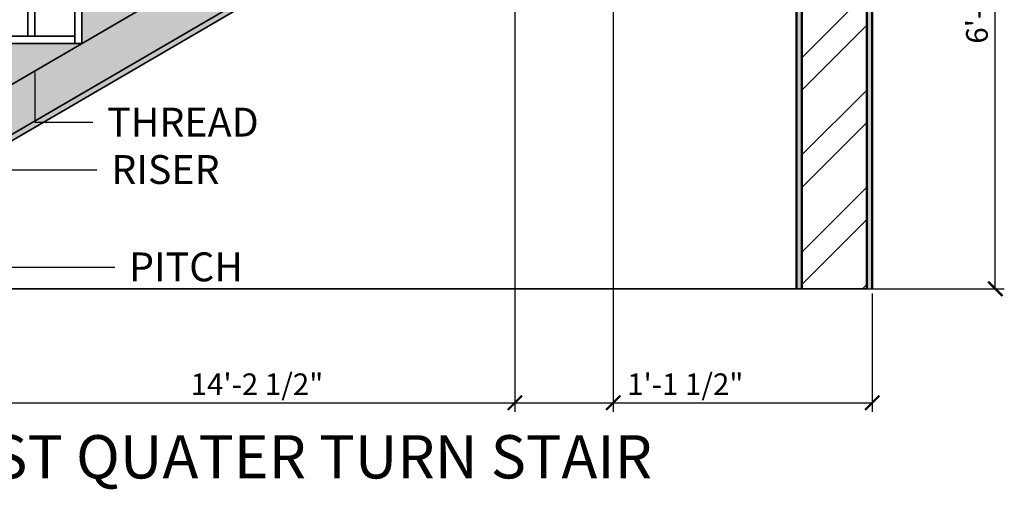
# Model space of a CAD drawing. Units: inches. Extents: x 2205 to 2524, y 4609 to 4803.
# Tile 2 of 5: x 2311 to 2447, y 4609 to 4674. Entities that reach past the tile are written whole.
import ezdxf
from ezdxf import colors
from ezdxf.entities.mleader import LeaderData, LeaderLine
from ezdxf.math import Vec2, Vec3

# ---------------------------------------------------------------- set-up
doc = ezdxf.new("R2010")
doc.units = ezdxf.units.IN
for name, color, linetype, lineweight in [('A-ANNO-DIMS', 2, 'Continuous', 18), ('A-ANNO-SYMB', 3, 'Continuous', 18), ('A-ANNO-TEXT', 7, 'Continuous', 18), ('A-FLOR-STRS', 7, 'Continuous', 35), ('A-SECT', 7, 'Continuous', 25), ('A-SECT-PATT', 252, 'Continuous', 13), ('A-WALL', 1, 'Continuous', 50), ('A-WALL-PATT', 8, 'Continuous', 13)]:
    doc.layers.add(name, color=color, linetype=linetype, lineweight=lineweight)
doc.styles.get("Standard").update_dxf_attribs({"font": 'arial.ttf'})
doc.dimstyles.new('ISO-25', dxfattribs={"dimtxt": 3, "dimasz": 2, "dimexe": 1.25, "dimexo": 0.625, "dimtad": 1, "dimdec": 1, "dimlunit": 3, "dimtxsty": 'Standard', "dimblk": 'ARCHTICK', "dimcen": 2.5, "dimclrd": 5, "dimclre": 2, "dimclrt": 6, "dimadec": 0, "dimazin": 0, "dimtfac": 1, "dimtdec": 1, "dimtmove": 0, "dimatfit": 3, "dimfxl": 1, "dimarcsym": 0})

# ---------------------------------------------------------------- blocks, each defined once
blk = doc.blocks.new('STAIR-STEP')
for p, q in [((2282.7, 4650.98), (2270.7, 4650.98)), ((2283.7, 4649.98), (2270.7, 4649.98)), ((2270.7, 4649.98), (2270.7, 4642.98)), ((2271.7, 4649.98), (2271.7, 4642.98))]:
    blk.add_line(p, q)
blk.add_arc((2270.7, 4650.48), 0.5, 90, 270)
blk = doc.blocks.new('BALUSTER')
for p, q in [((2276.2, 4684.66), (2276.2, 4650.98)), ((2277.2, 4685.25), (2277.2, 4650.98))]:
    blk.add_line(p, q)
blk = doc.blocks.new('_ArchTick')
at = {"color": 0, "linetype": 'ByBlock', "const_width": 0.15}
blk.add_lwpolyline([(-0.5, -0.5), (0.5, 0.5)], dxfattribs=at)
blk = doc.blocks.new('*D15')
at = {"layer": 'A-ANNO-DIMS', "color": 2, "lineweight": -2, "transparency": 16777216}
for p, q in [((2258.7, 4636.35), (2258.7, 4619.93)), ((2429.2, 4636.35), (2429.2, 4619.93))]:
    blk.add_line(p, q, dxfattribs=at)
at = {"layer": 'A-ANNO-DIMS', "color": 5, "lineweight": -2, "transparency": 16777216}
blk.add_line((2258.7, 4621.18), (2429.2, 4621.18), dxfattribs=at)
at = {"layer": 'DEFPOINTS', "color": 0, "transparency": 16777216}
for p in [(2258.7, 4636.98), (2429.2, 4636.98), (2429.2, 4621.18)]:
    blk.add_point(p, dxfattribs=at)
at = {"layer": 'A-ANNO-DIMS', "color": 5, "lineweight": -2, "transparency": 16777216, "xscale": 2, "yscale": 2, "zscale": 2, "rotation": 180}
blk.add_blockref('_ArchTick', (2258.7, 4621.18), dxfattribs=at)
at = {"layer": 'A-ANNO-DIMS', "color": 5, "lineweight": -2, "transparency": 16777216, "xscale": 2, "yscale": 2, "zscale": 2}
blk.add_blockref('_ArchTick', (2429.2, 4621.18), dxfattribs=at)
at = {"layer": 'A-ANNO-DIMS', "color": 6, "transparency": 16777216, "insert": (2343.95, 4623.36), "char_height": 3, "attachment_point": 5}
blk.add_mtext('14\'-2 1/2"', dxfattribs=at)
blk = doc.blocks.new('*D16')
at = {"layer": 'A-ANNO-DIMS', "color": 2, "lineweight": -2, "transparency": 16777216}
for p, q in [((2428.57, 4771.26), (2222.09, 4771.26)), ((2428.57, 4636.98), (2222.09, 4636.98))]:
    blk.add_line(p, q, dxfattribs=at)
at = {"layer": 'A-ANNO-DIMS', "color": 5, "lineweight": -2, "transparency": 16777216}
blk.add_line((2223.34, 4636.98), (2223.34, 4771.26), dxfattribs=at)
at = {"layer": 'DEFPOINTS', "color": 0, "transparency": 16777216}
for p in [(2223.34, 4771.26), (2429.2, 4771.26), (2429.2, 4636.98)]:
    blk.add_point(p, dxfattribs=at)
at = {"layer": 'A-ANNO-DIMS', "color": 5, "lineweight": -2, "transparency": 16777216, "xscale": 2, "yscale": 2, "zscale": 2}
for p, rotation in [((2223.34, 4771.26), 90), ((2223.34, 4636.98), 270)]:
    blk.add_blockref('_ArchTick', p, dxfattribs=dict(at, rotation=rotation))
at = {"layer": 'A-ANNO-DIMS', "color": 6, "transparency": 16777216, "insert": (2221.17, 4704.12), "char_height": 3, "attachment_point": 5, "rotation": 90}
blk.add_mtext('11\'-2 1/2"', dxfattribs=at)
blk = doc.blocks.new('*D17')
at = {"layer": 'A-ANNO-DIMS', "color": 2, "lineweight": -2, "transparency": 16777216}
for p, q in [((2420.07, 4713.98), (2447.5, 4713.98)), ((2420.07, 4636.98), (2447.5, 4636.98))]:
    blk.add_line(p, q, dxfattribs=at)
at = {"layer": 'A-ANNO-DIMS', "color": 5, "lineweight": -2, "transparency": 16777216}
blk.add_line((2446.25, 4636.98), (2446.25, 4713.98), dxfattribs=at)
at = {"layer": 'DEFPOINTS', "color": 0, "transparency": 16777216}
for p in [(2419.45, 4713.98), (2446.25, 4713.98), (2419.45, 4636.98)]:
    blk.add_point(p, dxfattribs=at)
at = {"layer": 'A-ANNO-DIMS', "color": 5, "lineweight": -2, "transparency": 16777216, "xscale": 2, "yscale": 2, "zscale": 2}
for p, rotation in [((2446.25, 4713.98), 90), ((2446.25, 4636.98), 270)]:
    blk.add_blockref('_ArchTick', p, dxfattribs=dict(at, rotation=rotation))
at = {"layer": 'A-ANNO-DIMS', "color": 6, "transparency": 16777216, "insert": (2444.09, 4675.48), "char_height": 3, "attachment_point": 5, "rotation": 90}
blk.add_mtext('6\'-5"', dxfattribs=at)
blk = doc.blocks.new('*D21')
at = {"layer": 'A-ANNO-DIMS', "color": 2, "lineweight": -2, "transparency": 16777216}
for p, q in [((2379.7, 4705.35), (2379.7, 4619.93)), ((2393.32, 4706.35), (2393.32, 4619.93))]:
    blk.add_line(p, q, dxfattribs=at)
at = {"layer": 'A-ANNO-DIMS', "color": 5, "lineweight": -2, "transparency": 16777216}
for p, q in [((2379.7, 4621.18), (2393.32, 4621.18)), ((2393.32, 4621.18), (2411.25, 4621.18))]:
    blk.add_line(p, q, dxfattribs=at)
at = {"layer": 'DEFPOINTS', "color": 0, "transparency": 16777216}
for p in [(2393.32, 4706.98), (2379.7, 4705.98), (2393.32, 4621.18)]:
    blk.add_point(p, dxfattribs=at)
at = {"layer": 'A-ANNO-DIMS', "color": 5, "lineweight": -2, "transparency": 16777216, "xscale": 2, "yscale": 2, "zscale": 2, "rotation": 180}
blk.add_blockref('_ArchTick', (2379.7, 4621.18), dxfattribs=at)
at = {"layer": 'A-ANNO-DIMS', "color": 5, "lineweight": -2, "transparency": 16777216, "xscale": 2, "yscale": 2, "zscale": 2}
blk.add_blockref('_ArchTick', (2393.32, 4621.18), dxfattribs=at)
at = {"layer": 'A-ANNO-DIMS', "color": 6, "transparency": 16777216, "insert": (2403.29, 4623.36), "char_height": 3, "attachment_point": 5}
blk.add_mtext('1\'-1 1/2"', dxfattribs=at)

msp = doc.modelspace()

# ---------------------------------------------------------------- hatches: boundary and pattern name
at = {"layer": 'A-SECT-PATT'}
h = msp.add_hatch(dxfattribs=at)
h.set_pattern_fill('AR-CONC', color=256, scale=0.04)
h.paths.add_polyline_path([(2393.32, 4706.98), (2419.45, 4706.98), (2425.45, 4706.98), (2425.45, 4712.98), (2419.45, 4712.98), (2379.7, 4712.98), (2379.7, 4705.98), (2271.7, 4642.98), (2259.7, 4636.98), (2273.32, 4636.98)])
h.paths.add_polyline_path([(2343.7, 4684.98), (2331.7, 4684.98), (2331.7, 4677.98)], flags=16)
h.paths.add_polyline_path([(2331.7, 4677.98), (2319.7, 4677.98), (2319.7, 4670.98)], flags=16)
h.paths.add_polyline_path([(2319.7, 4670.98), (2307.7, 4670.98), (2307.7, 4663.98)], flags=16)
h.paths.add_polyline_path([(2307.7, 4663.98), (2295.7, 4663.98), (2295.7, 4656.98)], flags=16)
h.paths.add_polyline_path([(2295.7, 4656.98), (2283.7, 4656.98), (2283.7, 4649.98)], flags=16)
h.paths.add_polyline_path([(2283.7, 4649.98), (2271.7, 4649.98), (2271.7, 4642.98)], flags=17)
h.paths.add_polyline_path([(2271.7, 4642.98), (2259.7, 4642.98), (2259.7, 4636.98)], flags=17)
h.paths.add_polyline_path([(2379.7, 4705.98), (2367.7, 4705.98), (2367.7, 4698.98)], flags=16)
h.paths.add_polyline_path([(2367.7, 4698.98), (2355.7, 4698.98), (2355.7, 4691.98)], flags=16)
h.paths.add_polyline_path([(2419.45, 4706.98), (2393.32, 4706.98), (2273.32, 4636.98), (2274.81, 4636.98), (2393.52, 4706.23), (2419.45, 4706.23)], flags=17)
h.paths.add_polyline_path([(2419.45, 4706.23), (2418.7, 4706.23), (2418.7, 4636.98), (2419.45, 4636.98)], flags=16)
h.paths.add_polyline_path([(2429.2, 4771.26), (2428.45, 4771.26), (2428.45, 4636.98), (2429.2, 4636.98)])
h.paths.add_polyline_path([(2419.45, 4771.26), (2418.7, 4771.26), (2418.7, 4713.98), (2419.45, 4713.98)])
at = {"layer": 'A-WALL-PATT'}
h = msp.add_hatch(dxfattribs=at)
h.set_pattern_fill('ANSI32', color=256)
h.paths.add_polyline_path([(2428.45, 4771.26), (2419.45, 4771.26), (2419.45, 4712.98), (2425.45, 4712.98), (2425.45, 4706.98), (2419.45, 4706.98), (2419.45, 4636.98), (2428.45, 4636.98)])

# ---------------------------------------------------------------- linework, layer by layer
at = {"layer": 'A-FLOR-STRS'}
for p, q in [((2273.32, 4636.98), (2393.32, 4706.98)), ((2271.7, 4642.98), (2379.7, 4705.98)), ((2274.81, 4636.98), (2393.52, 4706.23))]:
    msp.add_line(p, q, dxfattribs=at)
at = {"layer": 'A-SECT'}
msp.add_line((2239.14, 4636.98), (2429.2, 4636.98), dxfattribs=at)
at = {"layer": 'A-WALL'}
for p, q in [((2428.45, 4771.26), (2428.45, 4636.98)), ((2429.2, 4771.26), (2429.2, 4636.98)), ((2419.45, 4706.98), (2419.45, 4636.98)), ((2418.7, 4706.23), (2418.7, 4636.98))]:
    msp.add_line(p, q, dxfattribs=at)

# ---------------------------------------------------------------- block references
at = {"layer": 'A-FLOR-STRS'}
for name, p in [('BALUSTER', (36, 21)), ('STAIR-STEP', (48, 28)), ('STAIR-STEP', (36, 21))]:
    msp.add_blockref(name, p, dxfattribs=at)

# ---------------------------------------------------------------- texts
at = {"layer": 'A-ANNO-TEXT', "insert": (2266.99, 4616.69), "char_height": 6, "attachment_point": 1}
msp.add_mtext_dynamic_manual_height_columns('{\\fArial|b1|i0|c0|p34;NEWEL POST QUATER TURN STAIR}', width=215.8477, gutter_width=12.5, heights=[0], dxfattribs=at)

# ---------------------------------------------------------------- dimensions: what is measured, and where the dimension line sits
at = {"layer": 'A-ANNO-DIMS'}
for base, p1, p2, picture, middle in [((2223.34, 4771.26), (2429.2, 4636.98), (2429.2, 4771.26), '*D16', (2221.17, 4704.12)), ((2446.25, 4713.98), (2419.45, 4636.98), (2419.45, 4713.98), '*D17', (2444.09, 4675.48))]:
    dim = msp.add_linear_dim(base=base, p1=p1, p2=p2, angle=90, dimstyle='ISO-25', override={"dimdec": 1, "dimlfac": 1, "dimrnd": 0, "dimzin": 1, "dimdsep": 46, "dimlunit": 4, "dimfrac": 2}, dxfattribs=at)
    dim.commit()
    dim.dimension.update_dxf_attribs({"geometry": picture, "text_midpoint": middle})
for base, p1, p2, picture, middle in [((2393.32, 4621.18), (2379.7, 4705.98), (2393.32, 4706.98), '*D21', (2403.29, 4623.36)), ((2429.2, 4621.18), (2258.7, 4636.98), (2429.2, 4636.98), '*D15', (2343.95, 4623.36))]:
    dim = msp.add_linear_dim(base=base, p1=p1, p2=p2, dimstyle='ISO-25', override={"dimdec": 1, "dimlfac": 1, "dimrnd": 0, "dimzin": 1, "dimdsep": 46, "dimlunit": 4, "dimfrac": 2}, dxfattribs=at)
    dim.commit()
    dim.dimension.update_dxf_attribs({"geometry": picture, "text_midpoint": middle})

# ---------------------------------------------------------------- leaders
at = {"layer": 'A-ANNO-SYMB'}
ml = msp.add_multileader_mtext('Standard', dxfattribs=at)
ml.set_content('THREAD', color=256)
ml.set_leader_properties()
ml.build(insert=Vec2(0, 0))
ctx = ml.context
ctx.base_point, ctx.plane_origin = Vec3(2321.2, 4660.08), Vec3(2313.2, 4670.98)
notes = []
notes.append((ctx, [(0, (1, 1, 0), (2313.2, 4660.08), (1, 0), 8, [(0, [(2313.2, 4670.98)], 0, [])])]))
ctx.mtext.insert, ctx.mtext.width, ctx.mtext.flow_direction = Vec3(2323.2, 4662.08), 46.9984, 5
ml = msp.add_multileader_mtext('Standard', dxfattribs=at)
ml.set_content('RISER', color=256)
ml.set_leader_properties()
ml.build(insert=Vec2(0, 0))
ctx = ml.context
ctx.base_point, ctx.plane_origin = Vec3(2321.78, 4653.48), Vec3(2283.7, 4653.48)
notes.append((ctx, [(0, (1, 1, 0), (2313.78, 4653.48), (1, 0), 8, [(0, [(2283.7, 4653.48)], 0, [])])]))
ctx.mtext.insert, ctx.mtext.width, ctx.mtext.flow_direction = Vec3(2323.78, 4655.51), 29.2708, 5
ml = msp.add_multileader_mtext('Standard', dxfattribs=at)
ml.set_content('PITCH', color=256)
ml.set_leader_properties()
ml.build(insert=Vec2(0, 0))
ctx = ml.context
ctx.base_point, ctx.plane_origin = Vec3(2324.24, 4639.99), Vec3(2302.57, 4639.99)
notes.append((ctx, [(0, (1, 1, 0), (2316.24, 4639.99), (1, 0), 8, [(0, [(2302.57, 4639.99)], 0, [])])]))
ctx.mtext.insert, ctx.mtext.flow_direction = Vec3(2326.24, 4642.02), 5
for ctx, leaders in notes:
    for number, flags, end, landing, length, lines in leaders:
        leader = LeaderData()
        leader.index, (leader.has_last_leader_line, leader.has_dogleg_vector, leader.attachment_direction) = number, flags
        leader.last_leader_point, leader.dogleg_vector, leader.dogleg_length = Vec3(end), Vec3(landing), length
        for number, points, colour, breaks in lines:
            line = LeaderLine()
            line.index, line.vertices, line.color, line.breaks = number, Vec3.list(points), colors.encode_raw_color(colour), breaks
            leader.lines.append(line)
        ctx.leaders.append(leader)

doc.saveas('drawing.dxf')
